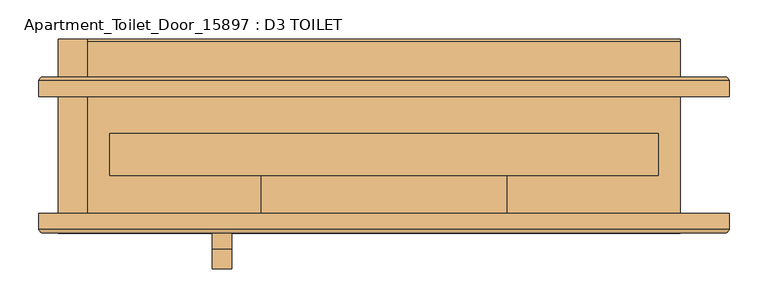
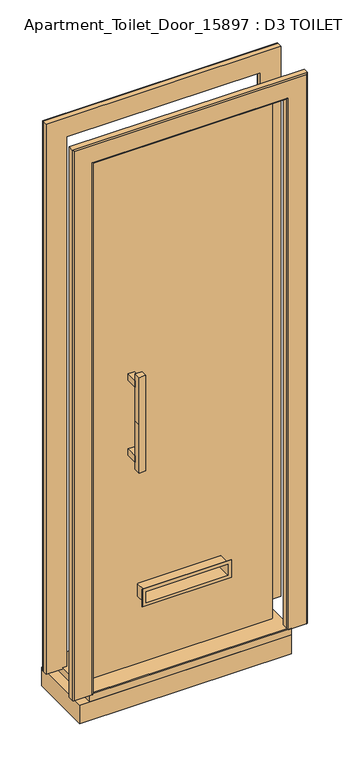
"""IFC4 building model written with IfcOpenShell, lengths in millimetres: door geometry, Apartment_Toilet_Door_15897 : D3 TOILET."""

from ifc_helpers import new_model, si_unit, frame, origin, place, context, project, spatial, polyline, circle_curve, ellipse_curve, outline, extrude, faceted_brep, source, transform, mapped, element, save
from ifc_brep_helpers import plane_surface, cylinder_surface, advanced_brep


def apartment_toilet_door_15897_d3_toilet_03746f18(model_context):
    return source(origin(), model_context, "Body", "SolidModel", [
        extrude(outline(polyline([(1241.0, -221.0), (1053.0132974, -221.0), (860.0, -221.0), (860.0, -196.0), (1050.7445158, -196.0), (1241.0, -196.0), (1241.0, -221.0)])), frame((0.0, -171.0, 0.0), z_axis=(0.0, 1.0, 0.0), x_axis=(0.0, 0.0, 1.0)), (0.0, 0.0, 1.0), 25.0),
        extrude(outline(polyline([(-196.0, -146.0), (-221.0, -146.0), (-221.0, -100.0), (-196.0, -100.0), (-196.0, -146.0)])), frame((0.0, 0.0, 1188.0), z_axis=(0.0, 0.0, 1.0), x_axis=(1.0, 0.0, 0.0)), (0.0, 0.0, 1.0), 25.0),
        extrude(outline(polyline([(-196.0, -146.0), (-221.0, -146.0), (-221.0, -100.0), (-196.0, -100.0), (-196.0, -146.0)])), frame((0.0, 0.0, 888.0), z_axis=(0.0, 0.0, 1.0), x_axis=(1.0, 0.0, 0.0)), (0.0, 0.0, 1.0), 25.0),
        extrude(outline(polyline([(-156.0, -46.0), (-251.0, -46.0), (-251.0, -42.0), (-156.0, -42.0), (-156.0, -46.0)])), frame((0.0, 0.0, 825.0), z_axis=(0.0, 0.0, 1.0), x_axis=(1.0, 0.0, 0.0)), (0.0, 0.0, 1.0), 451.0),
        extrude(outline(polyline([(2105.6000374, 353.0000374), (2105.6000374, -353.0000374), (5.0, -353.0000374), (5.0, 353.0000374), (2105.6000374, 353.0000374)]), holes=[polyline([(325.0, 156.0), (275.0, 156.0), (275.0, -156.0), (325.0, -156.0), (325.0, 156.0)])]), frame((0.0, -50.8, 0.0), z_axis=(0.0, 1.0, 0.0), x_axis=(0.0, 0.0, 1.0)), (0.0, 0.0, 1.0), 54.0),
        advanced_brep(
        [(-370.9983436, -125.0, 0.0), (-438.9986597, -125.0, 0.0), (-443.9993919, -119.9992678, 0.0), (-443.9993919, -100.0, 0.0), (-366.0, -100.0, 0.0), (-366.0, -120.0016564, 0.0), (-366.0, -120.0016564, 2118.6), (-370.9983436, -125.0, 2123.5983436), (-366.0, -100.0, 2118.6), (-443.9993919, -100.0, 2196.5993919), (443.9993919, -100.0, 2196.5993919), (443.9993919, -100.0, 0.0), (366.0, -100.0, 0.0), (366.0, -100.0, 2118.6), (-443.9993919, -119.9992678, 2196.5993919), (-438.9986597, -125.0, 2191.5986597), (370.9983436, -125.0, 2123.5983436), (370.9983436, -125.0, 0.0), (438.9986597, -125.0, 0.0), (438.9986597, -125.0, 2191.5986597), (366.0, -120.0016564, 0.0), (366.0, -120.0016564, 2118.6), (443.9993919, -119.9992678, 0.0), (443.9993919, -119.9992678, 2196.5993919)],
        [
            (0, 1),
            (1, 2, circle_curve(frame((-438.9986597, -119.9992678, 0.0), z_axis=(0.0, 0.0, -1.0), x_axis=(-1.0, 0.0, 0.0)), 5.0007322)),
            (2, 3),
            (3, 4),
            (4, 5),
            (5, 0, circle_curve(frame((-370.9983436, -120.0016564, 0.0), z_axis=(0.0, 0.0, -1.0), x_axis=(-1.0, 0.0, 0.0)), 4.9983436)),
            (5, 6),
            (6, 7, ellipse_curve(frame((-370.9983436, -120.0016564, 2123.5983436), z_axis=(-0.7071067811865475, 0.0, -0.7071067811865475), x_axis=(0.7071067811865474, 0.0, -0.7071067811865476)), 7.0687253, 4.9983436)),
            (7, 0),
            (4, 8),
            (8, 6),
            (3, 9),
            (9, 10),
            (10, 11),
            (11, 12),
            (12, 13),
            (13, 8),
            (2, 14),
            (14, 9),
            (1, 15),
            (15, 14, ellipse_curve(frame((-438.9986597, -119.9992678, 2191.5986597), z_axis=(-0.7071067811865475, 0.0, -0.7071067811865475), x_axis=(0.7071067811865474, 0.0, -0.7071067811865476)), 7.0721032, 5.0007322)),
            (7, 16),
            (16, 17),
            (17, 18),
            (18, 19),
            (19, 15),
            (12, 20),
            (20, 21),
            (21, 13),
            (17, 20, circle_curve(frame((370.9983436, -120.0016564, 0.0), z_axis=(0.0, 0.0, -1.0), x_axis=(1.0, 0.0, 0.0)), 4.9983436)),
            (11, 22),
            (22, 18, circle_curve(frame((438.9986597, -119.9992678, 0.0), z_axis=(0.0, 0.0, -1.0), x_axis=(1.0, 0.0, 0.0)), 5.0007322)),
            (23, 22),
            (10, 23),
            (23, 19, ellipse_curve(frame((438.9986597, -119.9992678, 2191.5986597), z_axis=(0.7071067811865475, 0.0, -0.7071067811865475), x_axis=(0.7071067811865474, 0.0, 0.7071067811865476)), 7.0721032, 5.0007322)),
            (16, 21, ellipse_curve(frame((370.9983436, -120.0016564, 2123.5983436), z_axis=(0.7071067811865475, 0.0, -0.7071067811865475), x_axis=(0.7071067811865474, 0.0, 0.7071067811865476)), 7.0687253, 4.9983436)),
            (6, 21),
            (14, 23),
        ],
        [
            plane_surface(frame((-381.0, 125.0, 0.0), z_axis=(0.0, 0.0, -1.0), x_axis=(0.0, 1.0, 0.0))),
            cylinder_surface(frame((-370.9983436, -120.0016564, 0.0), z_axis=(0.0, 0.0, -1.0), x_axis=(-1.0, 0.0, 0.0)), 4.9983436),
            plane_surface(frame((-366.0, -120.0016564, 0.0), z_axis=(1.0, 0.0, 0.0), x_axis=(0.0, 0.0, 1.0))),
            plane_surface(frame((-366.0, -100.0, 0.0), z_axis=(0.0, 1.0, 0.0), x_axis=(0.0, 0.0, 1.0))),
            plane_surface(frame((-443.9993919, -100.0, 0.0), z_axis=(-1.0, 0.0, 0.0), x_axis=(0.0, 0.0, 1.0))),
            cylinder_surface(frame((-438.9986597, -119.9992678, 0.0), z_axis=(0.0, 0.0, -1.0), x_axis=(-1.0, 0.0, 0.0)), 5.0007322),
            plane_surface(frame((-438.9986597, -125.0, 0.0), z_axis=(0.0, -1.0, 0.0), x_axis=(0.0, 0.0, 1.0))),
            plane_surface(frame((366.0, -120.0016564, 2118.6), z_axis=(-1.0, 0.0, 0.0), x_axis=(0.0, 0.0, -1.0))),
            plane_surface(frame((381.0, 125.0, 0.0), z_axis=(0.0, 0.0, -1.0), x_axis=(0.0, 1.0, 0.0))),
            plane_surface(frame((443.9993919, -100.0, 2196.5993919), z_axis=(1.0, 0.0, 0.0), x_axis=(0.0, 0.0, -1.0))),
            cylinder_surface(frame((438.9986597, -119.9992678, 2133.6), z_axis=(0.0, 0.0, 1.0), x_axis=(1.0, 0.0, 0.0)), 5.0007322),
            cylinder_surface(frame((370.9983436, -120.0016564, 2133.6), z_axis=(0.0, 0.0, 1.0), x_axis=(1.0, 0.0, 0.0)), 4.9983436),
            cylinder_surface(frame((-381.0, -120.0016564, 2123.5983436), z_axis=(-1.0, 0.0, 0.0), x_axis=(0.0, 0.0, 1.0)), 4.9983436),
            plane_surface(frame((-366.0, -120.0016564, 2118.6), z_axis=(0.0, 0.0, -1.0), x_axis=(1.0, 0.0, 0.0))),
            plane_surface(frame((-443.9993919, -100.0, 2196.5993919), z_axis=(0.0, 0.0, 1.0), x_axis=(1.0, 0.0, 0.0))),
            cylinder_surface(frame((-381.0, -119.9992678, 2191.5986597), z_axis=(-1.0, 0.0, 0.0), x_axis=(0.0, 0.0, 1.0)), 5.0007322),
        ],
        [
            (0, [[1, 2, 3, 4, 5, 6]]),
            (1, [[7, 8, 9, -6]]),
            (2, [[10, 11, -7, -5]]),
            (3, [[12, 13, 14, 15, 16, 17, -10, -4]]),
            (4, [[18, 19, -12, -3]]),
            (5, [[20, 21, -18, -2]]),
            (6, [[-9, 22, 23, 24, 25, 26, -20, -1]]),
            (7, [[-16, 27, 28, 29]]),
            (8, [[30, -27, -15, 31, 32, -24]]),
            (9, [[33, -31, -14, 34]]),
            (10, [[-25, -32, -33, 35]]),
            (11, [[-28, -30, -23, 36]]),
            (12, [[37, -36, -22, -8]]),
            (13, [[-17, -29, -37, -11]]),
            (14, [[38, -34, -13, -19]]),
            (15, [[-26, -35, -38, -21]]),
        ],
    ),
        advanced_brep(
        [(-370.9983436, 75.8, 0.0), (-366.0, 70.8016564, 0.0), (-366.0, 50.8, 0.0), (-443.9993919, 50.8, 0.0), (-443.9993919, 70.7992678, 0.0), (-438.9986597, 75.8, 0.0), (-438.9986597, 75.8, 2191.5986597), (438.9986597, 75.8, 2191.5986597), (438.9986597, 75.8, 0.0), (370.9983436, 75.8, 0.0), (370.9983436, 75.8, 2123.5983436), (-370.9983436, 75.8, 2123.5983436), (-443.9993919, 70.7992678, 2196.5993919), (-443.9993919, 50.8, 2196.5993919), (-366.0, 50.8, 2118.6), (366.0, 50.8, 2118.6), (366.0, 50.8, 0.0), (443.9993919, 50.8, 0.0), (443.9993919, 50.8, 2196.5993919), (-366.0, 70.8016564, 2118.6), (443.9993919, 70.7992678, 0.0), (443.9993919, 70.7992678, 2196.5993919), (366.0, 70.8016564, 0.0), (366.0, 70.8016564, 2118.6)],
        [
            (0, 1, circle_curve(frame((-370.9983436, 70.8016564, 0.0), z_axis=(0.0, 0.0, -1.0), x_axis=(1.0, 0.0, 0.0)), 4.9983436)),
            (1, 2),
            (2, 3),
            (3, 4),
            (4, 5, circle_curve(frame((-438.9986597, 70.7992678, 0.0), z_axis=(0.0, 0.0, -1.0), x_axis=(1.0, 0.0, 0.0)), 5.0007322)),
            (5, 0),
            (5, 6),
            (6, 7),
            (7, 8),
            (8, 9),
            (9, 10),
            (10, 11),
            (11, 0),
            (4, 12),
            (12, 6, ellipse_curve(frame((-438.9986597, 70.7992678, 2191.5986597), z_axis=(-0.7071067811865475, 0.0, -0.7071067811865475), x_axis=(0.7071067811865474, 0.0, -0.7071067811865476)), 7.0721032, 5.0007322)),
            (3, 13),
            (13, 12),
            (2, 14),
            (14, 15),
            (15, 16),
            (16, 17),
            (17, 18),
            (18, 13),
            (1, 19),
            (19, 14),
            (11, 19, ellipse_curve(frame((-370.9983436, 70.8016564, 2123.5983436), z_axis=(-0.7071067811865475, 0.0, -0.7071067811865475), x_axis=(0.7071067811865474, 0.0, -0.7071067811865476)), 7.0687253, 4.9983436)),
            (17, 20),
            (20, 21),
            (21, 18),
            (8, 20, circle_curve(frame((438.9986597, 70.7992678, 0.0), z_axis=(0.0, 0.0, -1.0), x_axis=(-1.0, 0.0, 0.0)), 5.0007322)),
            (16, 22),
            (22, 9, circle_curve(frame((370.9983436, 70.8016564, 0.0), z_axis=(0.0, 0.0, -1.0), x_axis=(-1.0, 0.0, 0.0)), 4.9983436)),
            (23, 22),
            (15, 23),
            (23, 10, ellipse_curve(frame((370.9983436, 70.8016564, 2123.5983436), z_axis=(0.7071067811865475, 0.0, -0.7071067811865475), x_axis=(0.7071067811865474, 0.0, 0.7071067811865476)), 7.0687253, 4.9983436)),
            (7, 21, ellipse_curve(frame((438.9986597, 70.7992678, 2191.5986597), z_axis=(0.7071067811865475, 0.0, -0.7071067811865475), x_axis=(0.7071067811865474, 0.0, 0.7071067811865476)), 7.0721032, 5.0007322)),
            (23, 19),
            (21, 12),
        ],
        [
            plane_surface(frame((-381.0, -125.0, 0.0), z_axis=(0.0, 0.0, -1.0), x_axis=(0.0, -1.0, 0.0))),
            plane_surface(frame((-370.9983436, 75.8, 0.0), z_axis=(0.0, 1.0, 0.0), x_axis=(0.0, 0.0, 1.0))),
            cylinder_surface(frame((-438.9986597, 70.7992678, 0.0), z_axis=(0.0, 0.0, -1.0), x_axis=(1.0, 0.0, 0.0)), 5.0007322),
            plane_surface(frame((-443.9993919, 70.7992678, 0.0), z_axis=(-1.0, 0.0, 0.0), x_axis=(0.0, 0.0, 1.0))),
            plane_surface(frame((-443.9993919, 50.8, 0.0), z_axis=(0.0, -1.0, 0.0), x_axis=(0.0, 0.0, 1.0))),
            plane_surface(frame((-366.0, 50.8, 0.0), z_axis=(1.0, 0.0, 0.0), x_axis=(0.0, 0.0, 1.0))),
            cylinder_surface(frame((-370.9983436, 70.8016564, 0.0), z_axis=(0.0, 0.0, -1.0), x_axis=(1.0, 0.0, 0.0)), 4.9983436),
            plane_surface(frame((443.9993919, 70.7992678, 2196.5993919), z_axis=(1.0, 0.0, 0.0), x_axis=(0.0, 0.0, -1.0))),
            plane_surface(frame((381.0, -125.0, 0.0), z_axis=(0.0, 0.0, -1.0), x_axis=(0.0, -1.0, 0.0))),
            plane_surface(frame((366.0, 50.8, 2118.6), z_axis=(-1.0, 0.0, 0.0), x_axis=(0.0, 0.0, -1.0))),
            cylinder_surface(frame((370.9983436, 70.8016564, 2133.6), z_axis=(0.0, 0.0, 1.0), x_axis=(-1.0, 0.0, 0.0)), 4.9983436),
            cylinder_surface(frame((438.9986597, 70.7992678, 2133.6), z_axis=(0.0, 0.0, 1.0), x_axis=(-1.0, 0.0, 0.0)), 5.0007322),
            cylinder_surface(frame((-381.0, 70.8016564, 2123.5983436), z_axis=(-1.0, 0.0, 0.0), x_axis=(0.0, 0.0, -1.0)), 4.9983436),
            plane_surface(frame((-366.0, 50.8, 2118.6), z_axis=(0.0, 0.0, -1.0), x_axis=(1.0, 0.0, 0.0))),
            plane_surface(frame((-443.9993919, 70.7992678, 2196.5993919), z_axis=(0.0, 0.0, 1.0), x_axis=(1.0, 0.0, 0.0))),
            cylinder_surface(frame((-381.0, 70.7992678, 2191.5986597), z_axis=(-1.0, 0.0, 0.0), x_axis=(0.0, 0.0, -1.0)), 5.0007322),
        ],
        [
            (0, [[1, 2, 3, 4, 5, 6]]),
            (1, [[7, 8, 9, 10, 11, 12, 13, -6]]),
            (2, [[14, 15, -7, -5]]),
            (3, [[16, 17, -14, -4]]),
            (4, [[18, 19, 20, 21, 22, 23, -16, -3]]),
            (5, [[24, 25, -18, -2]]),
            (6, [[-13, 26, -24, -1]]),
            (7, [[-22, 27, 28, 29]]),
            (8, [[-10, 30, -27, -21, 31, 32]]),
            (9, [[33, -31, -20, 34]]),
            (10, [[-11, -32, -33, 35]]),
            (11, [[-28, -30, -9, 36]]),
            (12, [[-12, -35, 37, -26]]),
            (13, [[-37, -34, -19, -25]]),
            (14, [[-23, -29, 38, -17]]),
            (15, [[-38, -36, -8, -15]]),
        ],
    ),
        extrude(outline(polyline([(122.5, 5.0), (125.0, 2.5), (125.0, -25.0), (-125.0, -25.0), (-125.0, 2.5), (-122.5, 5.0), (122.5, 5.0)])), frame((-381.0, 0.0, 0.0), z_axis=(1.0, 0.0, 0.0), x_axis=(0.0, 1.0, 0.0)), (0.0, 0.0, 1.0), 762.0),
        extrude(outline(polyline([(-419.0, 125.0), (381.0, 125.0), (381.0, -125.0), (-419.0, -125.0), (-419.0, 125.0)])), frame((0.0, 0.0, -100.0), z_axis=(0.0, 0.0, 1.0), x_axis=(1.0, 0.0, 0.0)), (0.0, 0.0, 1.0), 75.0),
        faceted_brep([(168.0, -46.0, 265.0), (-168.0, -46.0, 265.0), (-168.0, -44.0, 265.0), (168.0, -44.0, 265.0), (158.0, -100.0, 275.0), (-158.0, -100.0, 275.0), (-158.0, -46.0, 275.0), (158.0, -46.0, 275.0), (168.0, -102.0, 265.0), (-168.0, -102.0, 265.0), (-168.0, -100.0, 265.0), (168.0, -100.0, 265.0), (155.0, -44.0, 278.0), (-155.0, -44.0, 278.0), (-155.0, -102.0, 278.0), (155.0, -102.0, 278.0), (-168.0, -46.0, 335.0), (168.0, -46.0, 335.0), (168.0, -44.0, 335.0), (-168.0, -44.0, 335.0), (-158.0, -100.0, 325.0), (158.0, -100.0, 325.0), (158.0, -46.0, 325.0), (-158.0, -46.0, 325.0), (-168.0, -102.0, 335.0), (168.0, -102.0, 335.0), (168.0, -100.0, 335.0), (-168.0, -100.0, 335.0), (-155.0, -44.0, 322.0), (155.0, -44.0, 322.0), (155.0, -102.0, 322.0), (-155.0, -102.0, 322.0)], [[[0, 1, 2, 3]], [[4, 5, 6, 7]], [[8, 9, 10, 11]], [[12, 13, 14, 15]], [[16, 17, 18, 19]], [[20, 21, 22, 23]], [[24, 25, 26, 27]], [[28, 29, 30, 31]], [[17, 0, 3, 18]], [[21, 4, 7, 22]], [[25, 8, 11, 26]], [[29, 12, 15, 30]], [[19, 18, 3, 2], [28, 13, 12, 29]], [[1, 16, 19, 2]], [[16, 1, 0, 17], [23, 22, 7, 6]], [[5, 20, 23, 6]], [[27, 26, 11, 10], [20, 5, 4, 21]], [[9, 24, 27, 10]], [[24, 9, 8, 25], [31, 30, 15, 14]], [[13, 28, 31, 14]]]),
    ])


if __name__ == "__main__":
    model = new_model("IFC4")
    model_context = context("Model", 3, world=origin())
    ifc_project = project(units=[si_unit("LENGTHUNIT", "METRE", prefix="MILLI")], contexts=[model_context])
    site = spatial("IfcSite", under=ifc_project)
    building = spatial("IfcBuilding", under=site)
    placement = place(None, origin())
    apartment_toilet_door_15897_d3_toilet_shape = apartment_toilet_door_15897_d3_toilet_03746f18(model_context)
    element("IfcDoor", 1, ObjectType="Apartment_Toilet_Door_15897 : D3 TOILET", at=placement, inside=building, context=model_context, shape_type="MappedRepresentation", body=[
        mapped(apartment_toilet_door_15897_d3_toilet_shape, transform((0.0, 0.0, 0.0), x_axis=(1.0, 0.0, 0.0), y_axis=(0.0, 1.0, 0.0), z_axis=(0.0, 0.0, 1.0))),
    ])
    save(model, "model.ifc")

# Revit data of these elements
# Type "Apartment_Toilet_Door_15897 : D3 TOILET"
#   Type Mark = "15"
#   Panel Type = ""
#   Location [instance default] = ""
#   Door Type = "Semi Solid Flushed Wooden Door Laminated on Boths Sides- Bathroom / Laundry"
#   Construction Type Id = "DOOR"
#   Analytic Construction = "Wooden"
#   Threshold Depth = 0' - 1.1811"
#   Thickness = 0' - 2.12598"
#   Thermal Resistance (R) = 2.58758 (h·ft²·°F)/BTU
#   Heat Transfer Coefficient (U) = 0.386456 BTU/(h·ft²·°F)
#   Height = 7' - 0"
#   Trim Projection Ext = 0' - 0.98425"
#   Trim Projection Int = 0' - 0.98425"
#   Width = 2' - 6"
#   Define Thermal Properties by = 1
#   Threshold Material = BEL-Threshold material-Marble
#   Visual Light Transmittance = 0
#   Solar Heat Gain Coefficient = 0
#   Function = (empty or 0)
#   Wall Closure = (empty or 0)
# Element 1 (IfcDoor, "Apartment_Toilet_Door_15897 : D3 TOILET")
#   Materials on its faces: "Default", "Metal - IR - Satin Chrome", "BEL-Threshold material-Marble", "BEL-Threshold material-Mortar"
# Materials
#   "BEL-Threshold material-Marble": colour RGB 197 197 199, transparency 0, Cost = 0
#   "Default": colour RGB 127 127 127, transparency 0, Cost = 0
#   "Metal - IR - Satin Chrome": colour RGB 244 244 244, transparency 0, Cost = 0
#   "BEL-Threshold material-Mortar": colour RGB 141 151 158, transparency 0, Cost = 0
